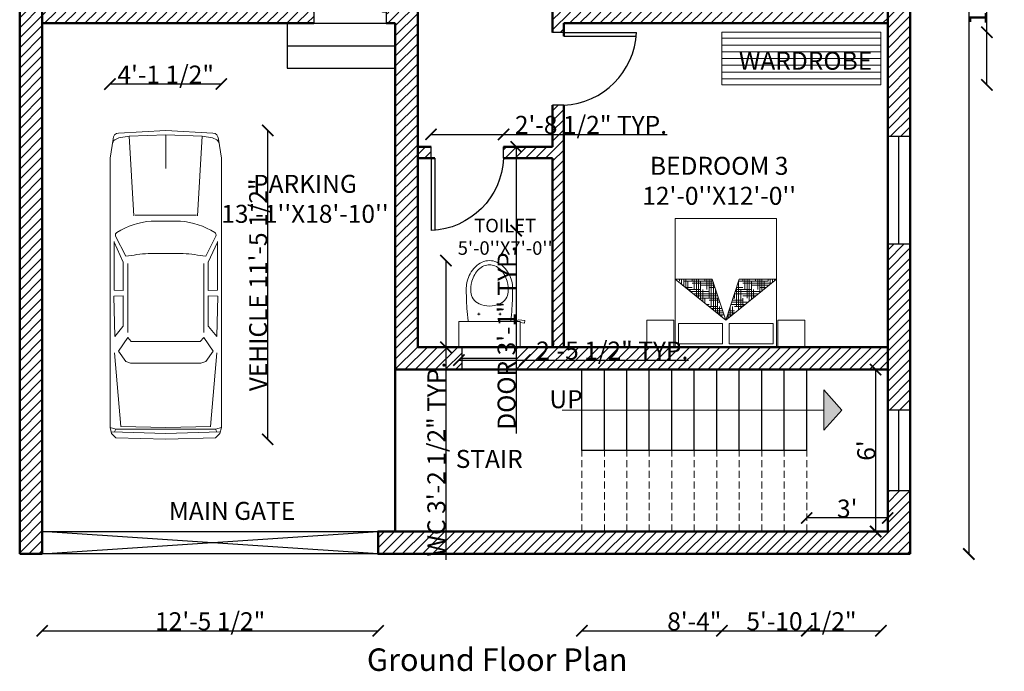
# Model space of a CAD drawing. Units: inches. Extents: x 1875 to 2385, y 1585 to 2263.
# Tile 1 of 3: x 1943 to 2381, y 1585 to 1875. Entities that reach past the tile are written whole.
import ezdxf

# ---------------------------------------------------------------- set-up
doc = ezdxf.new("R2010")
doc.units = ezdxf.units.IN
doc.header["$LTSCALE"] = 0.5
doc.linetypes.add('HIDDEN', pattern=[9.525, 6.35, -3.175])
for name, color, linetype, lineweight in [('A-ANNO-DIMS', 2, 'Continuous', 18), ('A-ANNO-SYMB', 50, 'Continuous', 18), ('A-ANNO-TEXT', 7, 'Continuous', 25), ('A-AREA-IDEN', 7, 'Continuous', 25), ('A-EQPM-VEHL', 8, 'Continuous', 18), ('A-FLOR-FIXT', 9, 'Continuous', 18), ('A-FLOR-STRS-HIDN', 50, 'HIDDEN', 18), ('A-FURN', 8, 'Continuous', 18), ('A-WALL-PATT', 8, 'Continuous', 13), ('Doors', 42, 'Continuous', 25), ('Entry', 10, 'Continuous', 25), ('Steps', 50, 'Continuous', 25), ('Walls', 7, 'Continuous', 50), ('Wardrobe', 202, 'Continuous', 18), ('Windows', 140, 'Continuous', 25)]:
    doc.layers.add(name, color=color, linetype=linetype, lineweight=lineweight)
doc.styles.get("Standard").update_dxf_attribs({"font": 'arial.ttf'})
doc.dimstyles.get("Standard").update_dxf_attribs({"dimtxt": 8, "dimasz": 5, "dimexe": 0.18, "dimexo": 0.0625, "dimgap": 0.09, "dimtad": 1, "dimdec": 1, "dimzin": 0, "dimdsep": 46, "dimlunit": 4, "dimtxsty": 'Standard', "dimblk": 'ARCHTICK', "dimcen": 0.09, "dimse1": 1, "dimse2": 1, "dimadec": 0, "dimazin": 0, "dimtfac": 1, "dimtdec": 1, "dimtofl": 0, "dimtmove": 0, "dimatfit": 3, "dimfxl": 1, "dimtolj": 1, "dimtzin": 0, "dimarcsym": 0})

# ---------------------------------------------------------------- blocks, each defined once
blk = doc.blocks.new('AP0B05')
for p, q in [((35, 100), (35, 880)), ((75, 100), (75, 879)), ((35, 100), (35, -20)), ((815, 100), (815, -20))]:
    blk.add_line(p, q)
blk.add_lwpolyline([(35, 100), (75, 100)])
blk.add_arc((-2, 63), 818, 2.6212, 87.3788)
blk = doc.blocks.new('02PCAR12')
at = {"color": 0, "linetype": 'ByBlock'}
for p, q in [((-210, 34), (-211, 0)), ((-207, 37), (-210, 34)), ((-203, 38), (-207, 37)), ((-206, 37), (-207, 0)), ((-204, 34.08), (-206, 35.08)), ((-203, 38.08), (-204, 34.08)), ((-204, -34), (-204, 34)), ((-19, 38), (-203, 38)), ((-202.36, 30.78), (-152, 35)), ((-113.23, 35.5), (-140.79, 34.89)), ((-140.79, 34.89), (-133.96, 29.23)), ((-113, 29), (-113.23, 35.5)), ((-109.42, 29.02), (-109.19, 35.33)), ((-109.19, 35.33), (-75.91, 35.3)), ((-76.45, 35.3), (-90, 29)), ((-72.15, 34.24), (-85.91, 27.37)), ((-6, 36), (-19, 38)), ((-5, 32), (-6.45, 34.89)), ((-202.36, 30.78), (-203, 0)), ((-157.9, 27.3), (-158.93, 24.08)), ((-150.83, 32.3), (-157.9, 27.3)), ((-141.48, 25.99), (-150.83, 32.3)), ((-134, 29), (-113, 29)), ((-90, 29), (-109.42, 29.02)), ((-5, 32), (-4, 25)), ((0, 0), (-1.8, 32.21)), ((-158.93, 24.08), (-158.93, -24)), ((-141.48, 25.99), (-144.24, 23.52)), ((-144.24, 23.52), (-144.24, 0)), ((-91, 26), (-138, 26)), ((-58.25, 21.76), (-4, 25)), ((-58, 0), (-58, 21)), ((-4, 25), (-3, 0)), ((-84, -12), (-84, 12)), ((-62, 10), (-62, 0)), ((-210, -34), (-211, 0)), ((-206, -37), (-207, 0)), ((-202.36, -30.78), (-203, 0)), ((-144.24, -23.52), (-144.24, 0)), ((-62, -10), (-62, 0)), ((-58, 0), (-58, -21)), ((-3, 0), (-26, 0)), ((-4, -25), (-3, 0)), ((0, 0), (-1.8, -32.21)), ((-157.9, -27.3), (-158.93, -24.08)), ((-141.48, -25.99), (-150.83, -32.3)), ((-141.48, -25.99), (-144.24, -23.52)), ((-91, -26), (-138, -26)), ((-58.25, -21.76), (-4, -25)), ((-5, -32), (-4, -25)), ((-202.36, -30.69), (-152, -34.92)), ((-150.83, -32.3), (-157.9, -27.3)), ((-140.79, -34.89), (-133.96, -29.23)), ((-134, -29), (-113, -29)), ((-113, -29), (-113.23, -35.5)), ((-90, -29), (-109.42, -29.02)), ((-109.42, -29.02), (-109.19, -35.33)), ((-76.45, -35.3), (-90, -29)), ((-72.15, -34.24), (-85.91, -27.37)), ((-5, -32), (-6.45, -34.89)), ((-207, -37), (-210, -34)), ((-203, -38), (-207, -37)), ((-204, -34), (-206, -35)), ((-203, -38), (-204, -34)), ((-19, -38), (-203, -38)), ((-113.23, -35.5), (-140.79, -34.89)), ((-109.19, -35.33), (-75.91, -35.3)), ((-6, -36), (-19, -38))]:
    blk.add_line(p, q, dxfattribs=at)
for centre, radius, start, end in [((-71.36, 32.4), 2, 31.5638, 113.12574), ((-8.24, 34), 2, 26.56505, 90), ((-5.8, 32), 4, 3.01279, 90), ((-461.05, -27.14), 379.08, 5.92644, 8.26698), ((-115.33, 5.39), 53.61, 4.93792, 31.5638), ((-461.05, 27.14), 379.08, 351.73302, 354.07356), ((-115.33, -5.39), 53.61, 328.4362, 355.06208), ((-71.36, -32.4), 2, 246.87426, 328.4362), ((-5.8, -32), 4, 270, 356.98721), ((-8.24, -34), 2, 270, 333.43495)]:
    blk.add_arc(centre, radius, start, end, dxfattribs=at)
blk = doc.blocks.new('*X4')
at = {"color": 0}
for p, q in [((20.149, 14.719), (20.277, 14.719)), ((20.156, 14.625), (20.156, 14.728)), ((20.174, 14.75), (20.277, 14.75)), ((20.188, 14.75), (20.188, 14.767)), ((20.199, 14.781), (20.277, 14.781)), ((20.25, 14.812), (20.277, 14.812)), ((20.25, 14.319), (20.25, 14.75)), ((20.031, 14.247), (20.031, 14.573)), ((20.062, 14.257), (20.062, 14.612)), ((20.094, 14.375), (20.094, 14.65)), ((20.098, 14.656), (20.125, 14.656)), ((20.124, 14.688), (20.25, 14.688)), ((20.125, 14.5), (20.125, 14.689)), ((20.125, 14.594), (20.277, 14.594)), ((20.219, 14.309), (20.219, 14.625)), ((20.25, 14.625), (20.277, 14.625)), ((19.922, 14.438), (20, 14.438)), ((19.948, 14.469), (20.125, 14.469)), ((19.973, 14.5), (20.25, 14.5)), ((19.998, 14.531), (20.277, 14.531)), ((20, 14.237), (20, 14.5)), ((20.023, 14.562), (20.277, 14.562)), ((20.188, 14.299), (20.188, 14.5)), ((20.25, 14.438), (20.277, 14.438)), ((19.797, 14.281), (20.125, 14.281)), ((19.812, 14.174), (19.812, 14.301)), ((19.822, 14.312), (20.229, 14.312)), ((19.844, 14.185), (19.844, 14.34)), ((19.875, 14.25), (19.875, 14.379)), ((19.875, 14.344), (20.277, 14.344)), ((19.906, 14.375), (19.906, 14.417)), ((19.969, 14.226), (19.969, 14.375)), ((20, 14.375), (20.277, 14.375)), ((20.125, 14.406), (20.277, 14.406)), ((20.156, 14.288), (20.156, 14.375)), ((19.721, 14.188), (19.75, 14.188)), ((19.746, 14.219), (19.875, 14.219)), ((19.75, 14.154), (19.75, 14.223)), ((19.772, 14.25), (20, 14.25)), ((19.781, 14.164), (19.781, 14.262)), ((19.938, 14.216), (19.938, 14.25)), ((19.702, 14.094), (19.779, 14.094)), ((19.719, 14.073), (19.719, 14.114)), ((19.727, 14.062), (19.873, 14.062)), ((19.75, 14.034), (19.75, 14.103)), ((19.752, 14.031), (19.875, 14.031)), ((19.781, 13.995), (19.781, 14.093)), ((19.812, 14), (19.812, 14.082)), ((19.875, 13.878), (19.875, 14)), ((19.906, 13.84), (19.906, 14.051)), ((19.938, 13.801), (19.938, 14.041)), ((19.969, 13.875), (19.969, 14.031)), ((20, 14), (20, 14.02)), ((20, 14), (20.061, 14)), ((20.062, 13.645), (20.062, 14)), ((20.094, 13.625), (20.094, 13.989)), ((19.827, 13.938), (20.25, 13.938)), ((19.853, 13.906), (20.125, 13.906)), ((19.875, 13.969), (20.156, 13.969)), ((19.878, 13.875), (20, 13.875)), ((20.031, 13.684), (20.031, 13.875)), ((20.125, 13.75), (20.125, 13.979)), ((20.125, 13.844), (20.277, 13.844)), ((20.156, 13.875), (20.156, 13.969)), ((20.219, 13.451), (20.219, 13.875)), ((20.25, 13.5), (20.25, 13.937)), ((20.25, 13.875), (20.277, 13.875)), ((19.953, 13.781), (20.277, 13.781)), ((19.978, 13.75), (20.25, 13.75)), ((20, 13.812), (20.277, 13.812)), ((20, 13.723), (20, 13.75)), ((20.003, 13.719), (20.125, 13.719)), ((20.188, 13.49), (20.188, 13.75)), ((20.079, 13.625), (20.277, 13.625)), ((20.104, 13.594), (20.277, 13.594)), ((20.125, 13.656), (20.277, 13.656)), ((20.129, 13.562), (20.25, 13.562)), ((20.156, 13.529), (20.156, 13.625)), ((20.25, 13.688), (20.277, 13.688)), ((20.205, 13.469), (20.277, 13.469)), ((20.23, 13.438), (20.277, 13.438)), ((20.25, 13.5), (20.277, 13.5)), ((20.255, 13.406), (20.277, 13.406))]:
    blk.add_line(p, q, dxfattribs=at)
blk = doc.blocks.new('MAT-P13')
for p, q in [((-1.17, 0), (-1.17, -0.4)), ((-1.17, 0), (-0.77, 0)), ((-0.77, 0), (-0.77, -0.4)), ((-0.75, 0), (0.75, 0)), ((-0.75, 0), (-0.75, -1.9)), ((0.75, 0), (0.75, -1.9)), ((0.77, 0), (1.17, 0)), ((0.77, 0), (0.77, -0.4)), ((1.17, 0), (1.17, -0.4)), ((-0.7, -0.05), (-0.7, -0.35)), ((-0.7, -0.05), (-0.05, -0.05)), ((-0.05, -0.35), (-0.05, -0.05)), ((0.05, -0.05), (0.7, -0.05)), ((0.05, -0.35), (0.05, -0.05)), ((0.7, -0.05), (0.7, -0.35)), ((-1.17, -0.4), (-0.77, -0.4)), ((-0.75, -1.003), (0, -0.4)), ((0, -0.4), (-0.75, -1.003)), ((-0.7, -0.35), (-0.05, -0.35)), ((0, -0.4), (-0.2, -1.003)), ((0, -0.4), (0.2, -1.003)), ((0, -0.4), (0.75, -1.003)), ((0.05, -0.35), (0.7, -0.35)), ((0.77, -0.4), (1.17, -0.4)), ((-0.75, -1.003), (-0.2, -1.003)), ((0.2, -1.003), (0.75, -1.003)), ((0.75, -1.9), (-0.75, -1.9))]:
    blk.add_line(p, q)
at = {"xscale": -1, "rotation": 90}
blk.add_blockref('*X4', (14.128, 19.274), dxfattribs=at)
blk = doc.blocks.new('toilet-1')
at = {"color": 0, "linetype": 'ByBlock'}
for p, q in [((-0.23, -0.02), (-0.23, -0.2116)), ((0.23, -0.02), (-0.23, -0.02)), ((0.23, -0.02), (0.23, -0.2116)), ((-0.23, -0.2116), (0.23, -0.2116)), ((0.1917, -0.2144), (0.2206, -0.225)), ((0.2206, -0.225), (0.266, -0.2187)), ((0.2633, -0.1997), (0.23, -0.2044)), ((0.266, -0.2187), (0.2633, -0.1997)), ((-0.0889, -0.2683), (-0.0697, -0.2683)), ((-0.0793, -0.2587), (-0.0793, -0.2778)), ((0.0889, -0.2683), (0.0698, -0.2683)), ((0.0794, -0.2587), (0.0794, -0.2778)), ((0, -0.6382), (0, -0.6382))]:
    blk.add_line(p, q, dxfattribs=at)
for centre, radius, start, end in [((3.5272, -0.6239), 3.7093, 173.69251, 175.15926), ((-3.527, -0.624), 3.7093, 4.84131, 6.31706), ((1.7368, -0.4519), 1.9109, 175.76982, 180.37578), ((-0.0312, -0.4465), 0.1114, 113.89968, 145.1485), ((0, -0.5169), 0.1884, 66.09393, 113.90607), ((0.0312, -0.4465), 0.1114, 34.8515, 66.10032), ((-1.7366, -0.4519), 1.9109, 359.62422, 4.23018), ((0.0981, -0.4497), 0.2389, 175.88621, 195.59308), ((-0.0408, -0.4398), 0.0996, 145.14967, 175.88096), ((0.0409, -0.4398), 0.0996, 4.11904, 34.85033), ((-0.098, -0.4497), 0.2389, 344.40692, 4.11379), ((0.0353, -0.463), 0.2093, 180.37466, 194.33753), ((0.055, -0.458), 0.2297, 194.33532, 209.62204), ((0.0961, -0.4503), 0.2369, 195.59686, 209.37705), ((-0.096, -0.4503), 0.2369, 330.62295, 344.40314), ((-0.0548, -0.458), 0.2297, 330.37879, 345.66551), ((-0.0351, -0.463), 0.2093, 345.6614, 359.62427), ((0.0647, -0.4524), 0.2409, 209.62726, 224.54888), ((0.0232, -0.4913), 0.1532, 209.38715, 226.54376), ((-0.0231, -0.4913), 0.1532, 313.45624, 330.61285), ((-0.0645, -0.4524), 0.2409, 315.45042, 330.37204), ((0.0178, -0.4986), 0.1751, 224.55199, 245.714), ((0.0152, -0.4997), 0.1416, 226.55015, 246.55272), ((0.0004, -0.538), 0.132, 245.58449, 269.87817), ((0, -0.5347), 0.1034, 246.54933, 270.0042), ((0, -0.5347), 0.1034, 269.9958, 293.45067), ((-0.0002, -0.538), 0.132, 270.12162, 294.4153), ((-0.0151, -0.4997), 0.1416, 293.44728, 313.44985), ((-0.0176, -0.4986), 0.1751, 294.28649, 315.4485)]:
    blk.add_arc(centre, radius, start, end, dxfattribs=at)
blk = doc.blocks.new('_ArchTick')
at = {"color": 0, "linetype": 'ByBlock', "const_width": 0.15}
blk.add_lwpolyline([(-0.5, -0.5), (0.5, 0.5)], dxfattribs=at)
blk = doc.blocks.new('*D13')
at = {"layer": 'A-ANNO-DIMS', "color": 0, "lineweight": -2, "ltscale": 0.5, "transparency": 16777216}
blk.add_line((2365.35, 2201.46), (2365.35, 1637.46), dxfattribs=at)
at = {"layer": 'Defpoints', "color": 0, "ltscale": 0.5, "transparency": 16777216}
for p in [(2339.28, 2201.46), (2339.28, 1637.46), (2365.35, 1637.46)]:
    blk.add_point(p, dxfattribs=at)
at = {"layer": 'A-ANNO-DIMS', "color": 0, "lineweight": -2, "ltscale": 0.5, "transparency": 16777216, "xscale": 5, "yscale": 5, "zscale": 5}
for p, rotation in [((2365.35, 2201.46), 90), ((2365.35, 1637.46), 270)]:
    blk.add_blockref('_ArchTick', p, dxfattribs=dict(at, rotation=rotation))
at = {"layer": 'A-ANNO-DIMS', "color": 0, "ltscale": 0.5, "transparency": 16777216, "insert": (2361.26, 1919.46), "char_height": 8, "attachment_point": 5, "rotation": 90}
blk.add_mtext("\\A1;47'", dxfattribs=at)
blk = doc.blocks.new('*D14')
at = {"layer": 'A-ANNO-DIMS', "color": 0, "lineweight": -2, "ltscale": 0.5, "transparency": 16777216}
blk.add_line((2323.92, 1719.46), (2323.92, 1647.46), dxfattribs=at)
at = {"layer": 'Defpoints', "color": 0, "ltscale": 0.5, "transparency": 16777216}
for p in [(2329.28, 1719.46), (2323.92, 1647.46), (2329.28, 1647.46)]:
    blk.add_point(p, dxfattribs=at)
at = {"layer": 'A-ANNO-DIMS', "color": 0, "lineweight": -2, "ltscale": 0.5, "transparency": 16777216, "xscale": 5, "yscale": 5, "zscale": 5}
for p, rotation in [((2323.92, 1719.46), 90), ((2323.92, 1647.46), 270)]:
    blk.add_blockref('_ArchTick', p, dxfattribs=dict(at, rotation=rotation))
at = {"layer": 'A-ANNO-DIMS', "color": 0, "ltscale": 0.5, "transparency": 16777216, "insert": (2319.75, 1683.46), "char_height": 8, "attachment_point": 5, "rotation": 90}
blk.add_mtext("\\A1;6'", dxfattribs=at)
blk = doc.blocks.new('*D15')
at = {"layer": 'A-ANNO-DIMS', "color": 0, "lineweight": -2, "ltscale": 0.5, "transparency": 16777216}
blk.add_line((2329.28, 1653.46), (2293.28, 1653.46), dxfattribs=at)
at = {"layer": 'Defpoints', "color": 0, "ltscale": 0.5, "transparency": 16777216}
for p in [(2293.28, 1653.46), (2293.28, 1647.46), (2329.28, 1647.46)]:
    blk.add_point(p, dxfattribs=at)
at = {"layer": 'A-ANNO-DIMS', "color": 0, "lineweight": -2, "ltscale": 0.5, "transparency": 16777216, "xscale": 5, "yscale": 5, "zscale": 5, "rotation": 180}
blk.add_blockref('_ArchTick', (2293.28, 1653.46), dxfattribs=at)
at = {"layer": 'A-ANNO-DIMS', "color": 0, "lineweight": -2, "ltscale": 0.5, "transparency": 16777216, "xscale": 5, "yscale": 5, "zscale": 5}
blk.add_blockref('_ArchTick', (2329.28, 1653.46), dxfattribs=at)
at = {"layer": 'A-ANNO-DIMS', "color": 0, "ltscale": 0.5, "transparency": 16777216, "insert": (2311.28, 1657.64), "char_height": 8, "attachment_point": 5}
blk.add_mtext("\\A1;3'", dxfattribs=at)
blk = doc.blocks.new('WIN-48IN')
at = {"ltscale": 0.5}
blk.add_line((0, 0), (48, 0), dxfattribs=at)
blk.add_lwpolyline([(0, 5), (48, 5), (48, -5), (0, -5)], close=True, dxfattribs=at)
blk = doc.blocks.new('WIN-24IN')
at = {"ltscale": 0.5}
blk.add_line((0, 0), (24, 0), dxfattribs=at)
blk.add_lwpolyline([(0, 5), (24, 5), (24, -5), (0, -5)], close=True, dxfattribs=at)
blk = doc.blocks.new('*D20')
at = {"layer": 'A-ANNO-DIMS', "color": 0, "lineweight": -2, "ltscale": 0.5, "transparency": 16777216}
for p, q in [((2164.05, 1818.46), (2164.05, 1781.24)), ((2164.05, 1781.24), (2164.05, 1691.06))]:
    blk.add_line(p, q, dxfattribs=at)
at = {"layer": 'Defpoints', "color": 0, "ltscale": 0.5, "transparency": 16777216}
for p in [(2158.46, 1818.46), (2158.46, 1781.24), (2164.05, 1781.24)]:
    blk.add_point(p, dxfattribs=at)
at = {"layer": 'A-ANNO-DIMS', "color": 0, "lineweight": -2, "ltscale": 0.5, "transparency": 16777216, "xscale": 5, "yscale": 5, "zscale": 5}
for p, rotation in [((2164.05, 1818.46), 90), ((2164.05, 1781.24), 270)]:
    blk.add_blockref('_ArchTick', p, dxfattribs=dict(at, rotation=rotation))
at = {"layer": 'A-ANNO-DIMS', "color": 0, "ltscale": 0.5, "transparency": 16777216, "insert": (2159.81, 1733.65), "char_height": 8, "attachment_point": 5, "rotation": 90}
blk.add_mtext('\\A1;DOOR 3\'-1" TYP.', dxfattribs=at)
blk = doc.blocks.new('*D21')
at = {"layer": 'A-ANNO-DIMS', "color": 0, "lineweight": -2, "ltscale": 0.5, "transparency": 16777216}
for p, q in [((2126.2, 1824.04), (2158.46, 1824.04)), ((2158.46, 1824.04), (2231.18, 1824.04))]:
    blk.add_line(p, q, dxfattribs=at)
at = {"layer": 'Defpoints', "color": 0, "ltscale": 0.5, "transparency": 16777216}
for p in [(2158.46, 1824.04), (2126.2, 1818.46), (2158.46, 1818.46)]:
    blk.add_point(p, dxfattribs=at)
at = {"layer": 'A-ANNO-DIMS', "color": 0, "lineweight": -2, "ltscale": 0.5, "transparency": 16777216, "xscale": 5, "yscale": 5, "zscale": 5, "rotation": 180}
blk.add_blockref('_ArchTick', (2126.2, 1824.04), dxfattribs=at)
at = {"layer": 'A-ANNO-DIMS', "color": 0, "lineweight": -2, "ltscale": 0.5, "transparency": 16777216, "xscale": 5, "yscale": 5, "zscale": 5}
blk.add_blockref('_ArchTick', (2158.46, 1824.04), dxfattribs=at)
at = {"layer": 'A-ANNO-DIMS', "color": 0, "ltscale": 0.5, "transparency": 16777216, "insert": (2197.32, 1828.27), "char_height": 8, "attachment_point": 5}
blk.add_mtext('\\A1;2\'-8 1/2" TYP.', dxfattribs=at)
blk = doc.blocks.new('*D30')
at = {"layer": 'A-ANNO-DIMS', "color": 0, "lineweight": -2, "ltscale": 0.5, "transparency": 16777216}
for p, q in [((2132.81, 1767.93), (2132.81, 1729.46)), ((2132.81, 1729.46), (2132.81, 1634.82))]:
    blk.add_line(p, q, dxfattribs=at)
at = {"layer": 'Defpoints', "color": 0, "ltscale": 0.5, "transparency": 16777216}
for p in [(2138.58, 1767.93), (2132.81, 1729.46), (2138.58, 1729.46)]:
    blk.add_point(p, dxfattribs=at)
at = {"layer": 'A-ANNO-DIMS', "color": 0, "lineweight": -2, "ltscale": 0.5, "transparency": 16777216, "xscale": 5, "yscale": 5, "zscale": 5}
for p, rotation in [((2132.81, 1767.93), 90), ((2132.81, 1729.46), 270)]:
    blk.add_blockref('_ArchTick', p, dxfattribs=dict(at, rotation=rotation))
at = {"layer": 'A-ANNO-DIMS', "color": 0, "ltscale": 0.5, "transparency": 16777216, "insert": (2128.58, 1679.64), "char_height": 8, "attachment_point": 5, "rotation": 90}
blk.add_mtext('\\A1;WC 3\'-2 1/2" TYP.', dxfattribs=at)
blk = doc.blocks.new('*D31')
at = {"layer": 'A-ANNO-DIMS', "color": 0, "lineweight": -2, "ltscale": 0.5, "transparency": 16777216}
for p, q in [((2138.58, 1723.69), (2167.93, 1723.69)), ((2167.93, 1723.69), (2240.66, 1723.69))]:
    blk.add_line(p, q, dxfattribs=at)
at = {"layer": 'Defpoints', "color": 0, "ltscale": 0.5, "transparency": 16777216}
for p in [(2138.58, 1729.46), (2167.93, 1729.46), (2167.93, 1723.69)]:
    blk.add_point(p, dxfattribs=at)
at = {"layer": 'A-ANNO-DIMS', "color": 0, "lineweight": -2, "ltscale": 0.5, "transparency": 16777216, "xscale": 5, "yscale": 5, "zscale": 5, "rotation": 180}
blk.add_blockref('_ArchTick', (2138.58, 1723.69), dxfattribs=at)
at = {"layer": 'A-ANNO-DIMS', "color": 0, "lineweight": -2, "ltscale": 0.5, "transparency": 16777216, "xscale": 5, "yscale": 5, "zscale": 5}
blk.add_blockref('_ArchTick', (2167.93, 1723.69), dxfattribs=at)
at = {"layer": 'A-ANNO-DIMS', "color": 0, "ltscale": 0.5, "transparency": 16777216, "insert": (2206.8, 1727.92), "char_height": 8, "attachment_point": 5}
blk.add_mtext('\\A1;2\'-5 1/2" TYP.', dxfattribs=at)
blk = doc.blocks.new('*D32')
at = {"layer": 'A-ANNO-DIMS', "color": 0, "lineweight": -2, "ltscale": 0.5, "transparency": 16777216}
blk.add_line((2053.56, 1688.47), (2053.56, 1825.8), dxfattribs=at)
at = {"layer": 'Defpoints', "color": 0, "ltscale": 0.5, "transparency": 16777216}
for p in [(2032.96, 1825.8), (2053.56, 1825.8), (2032.96, 1688.47)]:
    blk.add_point(p, dxfattribs=at)
at = {"layer": 'A-ANNO-DIMS', "color": 0, "lineweight": -2, "ltscale": 0.5, "transparency": 16777216, "xscale": 5, "yscale": 5, "zscale": 5}
for p, rotation in [((2053.56, 1825.8), 90), ((2053.56, 1688.47), 270)]:
    blk.add_blockref('_ArchTick', p, dxfattribs=dict(at, rotation=rotation))
at = {"layer": 'A-ANNO-DIMS', "color": 0, "ltscale": 0.5, "transparency": 16777216, "insert": (2049.33, 1757.14), "char_height": 8, "attachment_point": 5, "rotation": 90}
blk.add_mtext('\\A1;VEHICLE 11\'-5 1/2"', dxfattribs=at)
blk = doc.blocks.new('*D33')
at = {"layer": 'A-ANNO-DIMS', "color": 0, "lineweight": -2, "ltscale": 0.5, "transparency": 16777216}
blk.add_line((2032.96, 1846.4), (1983.44, 1846.4), dxfattribs=at)
at = {"layer": 'Defpoints', "color": 0, "ltscale": 0.5, "transparency": 16777216}
for p in [(1983.44, 1846.4), (1983.44, 1825.8), (2032.96, 1825.8)]:
    blk.add_point(p, dxfattribs=at)
at = {"layer": 'A-ANNO-DIMS', "color": 0, "lineweight": -2, "ltscale": 0.5, "transparency": 16777216, "xscale": 5, "yscale": 5, "zscale": 5, "rotation": 180}
blk.add_blockref('_ArchTick', (1983.44, 1846.4), dxfattribs=at)
at = {"layer": 'A-ANNO-DIMS', "color": 0, "lineweight": -2, "ltscale": 0.5, "transparency": 16777216, "xscale": 5, "yscale": 5, "zscale": 5}
blk.add_blockref('_ArchTick', (2032.96, 1846.4), dxfattribs=at)
at = {"layer": 'A-ANNO-DIMS', "color": 0, "ltscale": 0.5, "transparency": 16777216, "insert": (2008.2, 1850.63), "char_height": 8, "attachment_point": 5}
blk.add_mtext('\\A1;4\'-1 1/2"', dxfattribs=at)
blk = doc.blocks.new('*D42')
at = {"layer": 'A-ANNO-DIMS', "color": 0, "lineweight": -2, "ltscale": 0.5, "transparency": 16777216}
blk.add_line((1953.28, 1603.31), (2102.69, 1603.31), dxfattribs=at)
at = {"layer": 'Defpoints', "color": 0, "ltscale": 0.5, "transparency": 16777216}
for p in [(1953.28, 1647.46), (2102.69, 1647.46), (2102.69, 1603.31)]:
    blk.add_point(p, dxfattribs=at)
at = {"layer": 'A-ANNO-DIMS', "color": 0, "lineweight": -2, "ltscale": 0.5, "transparency": 16777216, "xscale": 5, "yscale": 5, "zscale": 5, "rotation": 180}
blk.add_blockref('_ArchTick', (1953.28, 1603.31), dxfattribs=at)
at = {"layer": 'A-ANNO-DIMS', "color": 0, "lineweight": -2, "ltscale": 0.5, "transparency": 16777216, "xscale": 5, "yscale": 5, "zscale": 5}
blk.add_blockref('_ArchTick', (2102.69, 1603.31), dxfattribs=at)
at = {"layer": 'A-ANNO-DIMS', "color": 0, "ltscale": 0.5, "transparency": 16777216, "insert": (2027.99, 1607.54), "char_height": 8, "attachment_point": 5}
blk.add_mtext('\\A1;12\'-5 1/2"', dxfattribs=at)
blk = doc.blocks.new('*D43')
at = {"layer": 'A-ANNO-DIMS', "color": 0, "lineweight": -2, "ltscale": 0.5, "transparency": 16777216}
blk.add_line((2193.28, 1603.31), (2293.28, 1603.31), dxfattribs=at)
at = {"layer": 'Defpoints', "color": 0, "ltscale": 0.5, "transparency": 16777216}
for p in [(2193.28, 1647.46), (2293.28, 1647.46), (2293.28, 1603.31)]:
    blk.add_point(p, dxfattribs=at)
at = {"layer": 'A-ANNO-DIMS', "color": 0, "lineweight": -2, "ltscale": 0.5, "transparency": 16777216, "xscale": 5, "yscale": 5, "zscale": 5, "rotation": 180}
blk.add_blockref('_ArchTick', (2193.28, 1603.31), dxfattribs=at)
at = {"layer": 'A-ANNO-DIMS', "color": 0, "lineweight": -2, "ltscale": 0.5, "transparency": 16777216, "xscale": 5, "yscale": 5, "zscale": 5}
blk.add_blockref('_ArchTick', (2293.28, 1603.31), dxfattribs=at)
at = {"layer": 'A-ANNO-DIMS', "color": 0, "ltscale": 0.5, "transparency": 16777216, "insert": (2243.28, 1607.48), "char_height": 8, "attachment_point": 5}
blk.add_mtext('\\A1;8\'-4"', dxfattribs=at)
blk = doc.blocks.new('*D47')
at = {"layer": 'A-ANNO-DIMS', "color": 0, "lineweight": -2, "ltscale": 0.5, "transparency": 16777216}
blk.add_line((2255.55, 1603.31), (2326.3, 1603.31), dxfattribs=at)
at = {"layer": 'Defpoints', "color": 0, "ltscale": 0.5, "transparency": 16777216}
for p in [(2255.55, 1846.07), (2326.3, 1846.07), (2326.3, 1603.31)]:
    blk.add_point(p, dxfattribs=at)
at = {"layer": 'A-ANNO-DIMS', "color": 0, "lineweight": -2, "ltscale": 0.5, "transparency": 16777216, "xscale": 5, "yscale": 5, "zscale": 5, "rotation": 180}
blk.add_blockref('_ArchTick', (2255.55, 1603.31), dxfattribs=at)
at = {"layer": 'A-ANNO-DIMS', "color": 0, "lineweight": -2, "ltscale": 0.5, "transparency": 16777216, "xscale": 5, "yscale": 5, "zscale": 5}
blk.add_blockref('_ArchTick', (2326.3, 1603.31), dxfattribs=at)
at = {"layer": 'A-ANNO-DIMS', "color": 0, "ltscale": 0.5, "transparency": 16777216, "insert": (2290.92, 1607.54), "char_height": 8, "attachment_point": 5}
blk.add_mtext('\\A1;5\'-10 1/2"', dxfattribs=at)
blk = doc.blocks.new('*D48')
at = {"layer": 'A-ANNO-DIMS', "color": 0, "lineweight": -2, "ltscale": 0.5, "transparency": 16777216}
for p, q in [((2373.43, 1869.47), (2373.43, 1920.02)), ((2373.43, 1846.07), (2373.43, 1869.47))]:
    blk.add_line(p, q, dxfattribs=at)
at = {"layer": 'Defpoints', "color": 0, "ltscale": 0.5, "transparency": 16777216}
for p in [(2326.3, 1869.47), (2373.43, 1869.47), (2326.3, 1846.07)]:
    blk.add_point(p, dxfattribs=at)
at = {"layer": 'A-ANNO-DIMS', "color": 0, "lineweight": -2, "ltscale": 0.5, "transparency": 16777216, "xscale": 5, "yscale": 5, "zscale": 5}
for p, rotation in [((2373.43, 1869.47), 90), ((2373.43, 1846.07), 270)]:
    blk.add_blockref('_ArchTick', p, dxfattribs=dict(at, rotation=rotation))
at = {"layer": 'A-ANNO-DIMS', "color": 0, "ltscale": 0.5, "transparency": 16777216, "insert": (2369.21, 1897.24), "char_height": 8, "attachment_point": 5, "rotation": 90}
blk.add_mtext('\\A1;1\'-11 1/2"', dxfattribs=at)

msp = doc.modelspace()

# ---------------------------------------------------------------- hatches: boundary and pattern name
at = {"layer": 'A-ANNO-SYMB', "ltscale": 0.5, "transparency": 33554585}
h = msp.add_hatch(color=256, dxfattribs=at)
h.dxf.hatch_style = 1
h.paths.add_polyline_path([(2300.85, 1710.43), (2300.85, 1692.49), (2308.92, 1701.46)])
at = {"layer": 'A-WALL-PATT', "ltscale": 0.5, "transparency": 33554585}
h = msp.add_hatch(dxfattribs=at)
h.set_pattern_fill('ANSI31', color=256)
h.paths.add_polyline_path([(2120.28, 2055.12), (2115.28, 2055.12), (2115.28, 2053.46), (1953.28, 2053.46), (1953.28, 2048.46), (2120.28, 2048.46)])
h.paths.add_polyline_path([(2339.28, 2009.69), (2329.28, 2009.69), (2329.28, 1958.74), (2339.28, 1958.74)])
h.paths.add_polyline_path([(2140.01, 1729.46), (2138.58, 1729.46), (2120.28, 1729.46), (2120.28, 1988.46), (2115.28, 1988.46), (2115.28, 1878.46), (2106.32, 1878.46), (2106.32, 1878.42), (2106.32, 1873.46), (2110.28, 1873.46), (2110.28, 1719.46), (2140.01, 1719.46)])
h.paths.add_polyline_path([(2074.06, 1878.46), (1953.28, 1878.46), (1953.28, 1873.46), (2074.06, 1873.46)])
h.paths.add_polyline_path([(1953.28, 1938.92), (1943.28, 1938.92), (1943.28, 1637.46), (1953.28, 1637.46), (1953.28, 1647.46)])
h.paths.add_polyline_path([(2329.28, 1729.46), (2164.01, 1729.46), (2164.01, 1719.46), (2329.28, 1719.46)])
h.paths.add_polyline_path([(2185.28, 1837.05), (2180.28, 1837.05), (2180.28, 1818.46), (2158.46, 1818.46), (2158.46, 1813.46), (2180.28, 1813.46), (2180.28, 1729.46), (2185.28, 1729.46)])
h.paths.add_polyline_path([(2126.2, 1818.46), (2120.28, 1818.46), (2120.28, 1813.46), (2126.2, 1813.46), (2126.2, 1813.5)], flags=17)
h.paths.add_polyline_path([(2339.28, 1910.74), (2329.28, 1910.74), (2329.28, 1823.21), (2339.28, 1823.21)])
h.paths.add_polyline_path([(2339.28, 1775.21), (2329.28, 1775.21), (2329.28, 1701.57), (2339.28, 1701.57)])
h.paths.add_polyline_path([(2339.28, 1665.57), (2329.28, 1665.57), (2329.28, 1647.46), (2110.28, 1647.46), (2102.69, 1647.46), (2102.69, 1637.46), (2110.28, 1637.46), (2339.28, 1637.46)])
h = msp.add_hatch(dxfattribs=at)
h.set_pattern_fill('ANSI31', color=256)
h.paths.add_polyline_path([(2329.28, 1994.46), (2221.28, 1994.46), (2221.28, 1995.51), (2221.25, 1995.51), (2216.28, 1995.51), (2216.28, 1953.46), (2221.28, 1953.46), (2221.28, 1989.46), (2329.28, 1989.46)])
h.paths.add_polyline_path([(2221.28, 1914.46), (2216.28, 1914.46), (2216.28, 1878.46), (2180.28, 1878.46), (2180.28, 1869.31), (2185.28, 1869.31), (2185.28, 1873.46), (2329.28, 1873.46), (2329.28, 1878.46), (2221.28, 1878.46)])

# ---------------------------------------------------------------- linework, layer by layer
at = {"layer": 'A-ANNO-SYMB', "ltscale": 0.5}
for p, q in [((2300.85, 1710.43), (2300.85, 1692.49)), ((2308.92, 1701.46), (2300.85, 1710.43)), ((2184.47, 1701.46), (2300.85, 1701.46)), ((2308.92, 1701.46), (2300.85, 1692.49))]:
    msp.add_line(p, q, dxfattribs=at)
at = {"layer": 'A-FLOR-STRS-HIDN'}
for p, q in [((2193.28, 1647.46), (2193.28, 1683.46)), ((2203.28, 1647.46), (2203.28, 1683.46)), ((2213.28, 1647.46), (2213.28, 1683.46)), ((2223.28, 1647.46), (2223.28, 1683.46)), ((2233.28, 1647.46), (2233.28, 1683.46)), ((2243.28, 1647.46), (2243.28, 1683.46)), ((2253.28, 1647.46), (2253.28, 1683.46)), ((2263.28, 1647.46), (2263.28, 1683.46)), ((2273.28, 1647.46), (2273.28, 1683.46)), ((2283.28, 1647.46), (2283.28, 1683.46)), ((2293.28, 1647.46), (2293.28, 1683.46))]:
    msp.add_line(p, q, dxfattribs=at)
at = {"layer": 'Entry'}
for p, q in [((1953.28, 1637.46), (1953.28, 1647.46)), ((1953.28, 1647.46), (2102.69, 1647.46)), ((2102.69, 1637.46), (1953.28, 1647.46)), ((1953.28, 1637.46), (2102.69, 1647.46)), ((2102.69, 1647.46), (2102.69, 1637.46)), ((2102.69, 1637.46), (1953.28, 1637.46))]:
    msp.add_line(p, q, dxfattribs=at)
at = {"layer": 'Steps', "ltscale": 0.5}
for p, q in [((2062.28, 1873.46), (2062.28, 1853.46)), ((2062.28, 1873.46), (2110.28, 1873.46)), ((2062.28, 1863.46), (2110.28, 1863.46)), ((2062.28, 1853.46), (2110.28, 1853.46))]:
    msp.add_line(p, q, dxfattribs=at)
at = {"layer": 'Steps'}
for p, q in [((2193.28, 1683.46), (2193.28, 1719.46)), ((2203.28, 1683.46), (2203.28, 1719.46)), ((2213.28, 1683.46), (2213.28, 1719.46)), ((2223.28, 1683.46), (2223.28, 1719.46)), ((2233.28, 1683.46), (2233.28, 1719.46)), ((2243.28, 1683.46), (2243.28, 1719.46)), ((2253.28, 1683.46), (2253.28, 1719.46)), ((2263.28, 1683.46), (2263.28, 1719.46)), ((2273.28, 1683.46), (2273.28, 1719.46)), ((2283.28, 1683.46), (2283.28, 1719.46)), ((2293.28, 1683.46), (2293.28, 1719.46)), ((2293.28, 1683.46), (2193.28, 1683.46))]:
    msp.add_line(p, q, dxfattribs=at)
at = {"layer": 'Walls'}
for p, q in [((1943.28, 2201.46), (1943.28, 1637.46)), ((2339.28, 2201.46), (2339.28, 1637.46)), ((1953.28, 2191.46), (1953.28, 1637.46)), ((2329.28, 2191.46), (2329.28, 1647.46)), ((2120.28, 1988.46), (2120.28, 1729.46)), ((2180.28, 1878.46), (2180.28, 1869.31)), ((2180.28, 1878.46), (2180.28, 1869.31)), ((1953.28, 1873.46), (2074.06, 1873.46)), ((2106.32, 1873.46), (2110.28, 1873.46)), ((2110.28, 1873.46), (2110.28, 1647.46)), ((2185.28, 1873.46), (2329.28, 1873.46)), ((2185.28, 1873.46), (2185.28, 1867.66)), ((2180.28, 1837.05), (2180.28, 1818.46)), ((2180.28, 1837.05), (2180.28, 1818.46)), ((2185.28, 1837.05), (2185.28, 1729.46)), ((2120.28, 1818.46), (2126.2, 1818.46)), ((2158.46, 1818.46), (2180.28, 1818.46)), ((2120.28, 1813.46), (2127.86, 1813.46)), ((2158.46, 1813.46), (2180.28, 1813.46)), ((2180.28, 1813.46), (2180.28, 1729.46)), ((2180.28, 1813.46), (2180.28, 1794.46)), ((2120.28, 1729.46), (2329.28, 1729.46)), ((2110.28, 1719.46), (2329.28, 1719.46)), ((1943.28, 1637.46), (1953.28, 1637.46))]:
    msp.add_line(p, q, dxfattribs=at)
msp.add_lwpolyline([(2329.28, 1647.46), (2110.28, 1647.46), (2102.69, 1647.46), (2102.69, 1637.46), (2110.28, 1637.46), (2339.28, 1637.46)], dxfattribs=at)
at = {"layer": 'Wardrobe', "ltscale": 0.5}
for p, q in [((2255.55, 1866.77), (2326.3, 1866.77)), ((2255.55, 1863.77), (2326.3, 1863.77)), ((2255.55, 1860.77), (2326.3, 1860.77)), ((2255.55, 1857.77), (2326.3, 1857.77)), ((2255.55, 1854.77), (2326.3, 1854.77)), ((2255.55, 1851.77), (2326.3, 1851.77)), ((2255.55, 1848.77), (2326.3, 1848.77))]:
    msp.add_line(p, q, dxfattribs=at)
msp.add_lwpolyline([(2255.55, 1869.47), (2326.3, 1869.47), (2326.3, 1846.07), (2255.55, 1846.07)], close=True, dxfattribs=at)
at = {"layer": 'Windows', "ltscale": 0.5}
msp.add_line((2334.28, 1665.57), (2334.28, 1701.57), dxfattribs=at)
msp.add_lwpolyline([(2329.28, 1665.57), (2329.28, 1701.57), (2339.28, 1701.57), (2339.28, 1665.57)], close=True, dxfattribs=at)

# ---------------------------------------------------------------- block references
at = {"layer": 'A-EQPM-VEHL', "ltscale": 0.5, "xscale": 0.6508489368000642, "yscale": 0.6508489368000642, "zscale": 0.6508489368000642, "rotation": 90}
msp.add_blockref('02PCAR12', (2008.23, 1825.8), dxfattribs=at)
at = {"layer": 'A-FLOR-FIXT', "ltscale": 0.5, "xscale": -59.18137808131736, "yscale": 59.18137808131736, "zscale": 59.18137808131736, "rotation": 180}
msp.add_blockref('toilet-1', (2152.19, 1728.28), dxfattribs=at)
at = {"layer": 'A-FURN', "ltscale": 0.5, "xscale": -30.05916968857566, "yscale": 30.05916968857566, "zscale": 30.05916968857566, "rotation": 180}
msp.add_blockref('MAT-P13', (2257.28, 1729.46), dxfattribs=at)
at = {"layer": 'Doors', "xscale": -0.0413587909994788, "yscale": 0.0413587909994788, "zscale": 0.0413587909994788}
msp.add_blockref('AP0B05', (2107.76, 1874.29), dxfattribs=at)
at = {"layer": 'Doors', "yscale": 0.0413587909994788, "zscale": 0.0413587909994788}
for p, xscale, rotation in [((2181.11, 1870.76), 0.0413587909994788, 270), ((2124.76, 1817.63), -0.0413587909994788, 180)]:
    msp.add_blockref('AP0B05', p, dxfattribs=dict(at, xscale=xscale, rotation=rotation))
at = {"layer": 'Windows', "rotation": 89.99999999999818}
msp.add_blockref('WIN-48IN', (2334.28, 1775.21), dxfattribs=at)
at = {"layer": 'Windows'}
msp.add_blockref('WIN-24IN', (2140.01, 1724.46), dxfattribs=at)

# ---------------------------------------------------------------- texts
at = {"layer": 'A-ANNO-TEXT', "ltscale": 0.5}
msp.add_text('Ground Floor Plan', height=10, dxfattribs=at).set_placement((2097.69, 1585.46))
at = {"layer": 'A-ANNO-TEXT', "ltscale": 0.5, "char_height": 8, "attachment_point": 1}
for s, width, insert in [('\\pxqc;WARDROBE', 74.3766, (2255.55, 1860.77)), ('\\pxqc;UP', 22.1772, (2175.15, 1710.28)), ('\\pxqc;MAIN GATE', 74.3766, (2000.53, 1660.62))]:
    msp.add_mtext_dynamic_manual_height_columns(s, width=width, gutter_width=12.5, heights=[0], dxfattribs=dict(at, insert=insert))
at = {"layer": 'A-AREA-IDEN', "ltscale": 0.5, "attachment_point": 1}
for s, insert, char_height in [("\\pxqc;BEDROOM 3\\P12'-0''X12'-0''", (2217.16, 1814.06), 8), ("\\pxqc;PARKING\\P13'-1''X18'-10''", (2032.96, 1806.05), 8), ("\\pxqc;TOILET\\P5'-0''X7'-0''", (2121.99, 1786.5), 6), ('\\pxqc;STAIR', (2114.89, 1683.73), 8)]:
    msp.add_mtext_dynamic_manual_height_columns(s, width=74.3766, gutter_width=12.5, heights=[0], dxfattribs=dict(at, insert=insert, char_height=char_height))

# ---------------------------------------------------------------- dimensions: what is measured, and where the dimension line sits
at = {"layer": 'A-ANNO-DIMS', "ltscale": 0.5}
for base, p1, p2, angle, override, picture, middle in [((2365.35, 1637.46), (2339.28, 2201.46), (2339.28, 1637.46), 90, {"dimclrd": 0, "dimclre": 0, "dimclrt": 0}, '*D13', (2361.26, 1919.46)), ((2373.43, 1869.47), (2326.3, 1846.07), (2326.3, 1869.47), 90, {"dimdec": 1, "dimlfac": 1, "dimrnd": 0, "dimzin": 1, "dimdsep": 46, "dimlunit": 4, "dimfrac": 2}, '*D48', (2369.21, 1897.24)), ((1983.44, 1846.4), (2032.96, 1825.8), (1983.44, 1825.8), 180, {"dimdec": 1, "dimlfac": 1, "dimrnd": 0, "dimzin": 1, "dimdsep": 46, "dimlunit": 4, "dimfrac": 2}, '*D33', (2008.2, 1850.63)), ((2323.92, 1647.46), (2329.28, 1719.46), (2329.28, 1647.46), 90, {"dimclrd": 0, "dimclre": 0, "dimclrt": 0}, '*D14', (2319.75, 1683.46))]:
    dim = msp.add_linear_dim(base=base, p1=p1, p2=p2, angle=angle, dimstyle='Standard', override=override, dxfattribs=at)
    dim.commit()
    dim.dimension.update_dxf_attribs({"geometry": picture, "text_midpoint": middle})
for base, p1, p2, picture, middle in [((2158.46, 1824.04), (2126.2, 1818.46), (2158.46, 1818.46), '*D21', (2197.32, 1828.27)), ((2167.9344, 1723.6898), (2138.5803, 1729.46), (2167.9344, 1729.46), '*D31', (2206.7952, 1727.9162))]:
    dim = msp.add_linear_dim(base=base, p1=p1, p2=p2, text='<> TYP.', dimstyle='Standard', override={"dimdec": 1, "dimlfac": 1, "dimrnd": 0, "dimzin": 1, "dimdsep": 46, "dimlunit": 4, "dimfrac": 2}, dxfattribs=at)
    dim.commit()
    dim.dimension.update_dxf_attribs({"geometry": picture, "text_midpoint": middle})
for base, p1, p2, override, picture, middle in [((2326.2953, 1603.31), (2255.5527, 1846.0739), (2326.2953, 1846.0739), {"dimdec": 1, "dimlfac": 1, "dimrnd": 0, "dimzin": 1, "dimdsep": 46, "dimlunit": 4, "dimfrac": 2}, '*D47', (2290.924, 1607.5364)), ((2293.28, 1653.46), (2329.28, 1647.46), (2293.28, 1647.46), {"dimclrd": 0, "dimclre": 0, "dimclrt": 0}, '*D15', (2311.28, 1657.64)), ((2102.69, 1603.31), (1953.28, 1647.46), (2102.69, 1647.46), {"dimdec": 1, "dimlfac": 1, "dimrnd": 0, "dimzin": 1, "dimdsep": 46, "dimlunit": 4, "dimfrac": 2}, '*D42', (2027.99, 1607.54)), ((2293.28, 1603.31), (2193.28, 1647.46), (2293.28, 1647.46), {"dimdec": 1, "dimlfac": 1, "dimrnd": 0, "dimzin": 1, "dimdsep": 46, "dimlunit": 4, "dimfrac": 2}, '*D43', (2243.28, 1607.48))]:
    dim = msp.add_linear_dim(base=base, p1=p1, p2=p2, dimstyle='Standard', override=override, dxfattribs=at)
    dim.commit()
    dim.dimension.update_dxf_attribs({"geometry": picture, "text_midpoint": middle})
for base, p1, p2, angle, text, picture, middle in [((2053.56, 1825.8), (2032.96, 1688.47), (2032.96, 1825.8), 90, 'VEHICLE <>', '*D32', (2049.33, 1757.14)), ((2164.05, 1781.24), (2158.46, 1818.46), (2158.46, 1781.24), 270, 'DOOR <> TYP.', '*D20', (2159.81, 1733.65)), ((2132.81, 1729.46), (2138.58, 1767.93), (2138.58, 1729.46), 270, 'WC <> TYP.', '*D30', (2128.58, 1679.64))]:
    dim = msp.add_linear_dim(base=base, p1=p1, p2=p2, angle=angle, text=text, dimstyle='Standard', override={"dimdec": 1, "dimlfac": 1, "dimrnd": 0, "dimzin": 1, "dimdsep": 46, "dimlunit": 4, "dimfrac": 2}, dxfattribs=at)
    dim.commit()
    dim.dimension.update_dxf_attribs({"geometry": picture, "text_midpoint": middle})

doc.saveas('drawing.dxf')
